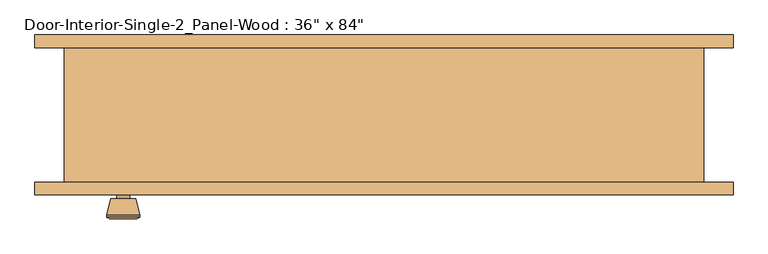
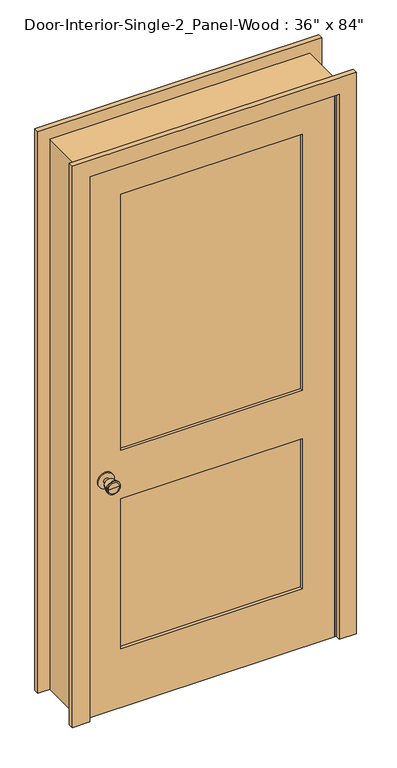
"""IFC4 building model written with IfcOpenShell, lengths in millimetres: door geometry."""

from ifc_helpers import new_model, si_unit, point, frame, frame_2d, origin, place, context, project, spatial, polyline, circle_curve, trimmed, segment, composite_curve, outline, extrude, faceted_brep, source, transform, mapped, element, save
from ifc_brep_helpers import plane_surface, cylinder_surface, revolved_surface, advanced_brep


def door_387d6dd4(model_context):
    return source(origin(), model_context, "Body", "SolidModel", [
        advanced_brep(
        [(-393.7, -57.5, 914.4), (-403.7, -57.5, 914.4), (-383.7, -57.5, 914.4), (-373.2241324, -8.5, 914.4), (-414.1758676, -8.5, 914.4), (-393.7, -8.5, 914.4), (-368.7, -10.3278681, 914.4), (-418.7, -10.3278681, 914.4), (-368.7, -13.7915463, 914.4), (-418.7, -13.7915463, 914.4), (-375.063764, -38.5, 914.4), (-412.336236, -38.5, 914.4), (-383.7, -38.5, 914.4), (-403.7, -38.5, 914.4)],
        [
            (0, 1),
            (1, 2, circle_curve(frame((-393.7, -57.5, 914.4), z_axis=(0.0, -1.0, 0.0), x_axis=(-1.0, 0.0, 0.0)), 10.0)),
            (2, 0),
            (2, 1, circle_curve(frame((-393.7, -57.5, 914.4), z_axis=(0.0, -1.0, 0.0), x_axis=(-1.0, 0.0, 0.0)), 10.0)),
            (3, 4, circle_curve(frame((-393.7, -8.5, 914.4), z_axis=(0.0, 1.0, 0.0), x_axis=(-1.0, 0.0, 0.0)), 20.4758676)),
            (4, 5),
            (5, 3),
            (4, 3, circle_curve(frame((-393.7, -8.5, 914.4), z_axis=(0.0, 1.0, 0.0), x_axis=(-1.0, 0.0, 0.0)), 20.4758676)),
            (6, 7, circle_curve(frame((-393.7, -10.3278681, 914.4), z_axis=(0.0, 1.0, 0.0), x_axis=(-1.0, 0.0, 0.0)), 25.0)),
            (7, 4),
            (3, 6),
            (7, 6, circle_curve(frame((-393.7, -10.3278681, 914.4), z_axis=(0.0, 1.0, 0.0), x_axis=(-1.0, 0.0, 0.0)), 25.0)),
            (8, 9, circle_curve(frame((-393.7, -13.7915463, 914.4), z_axis=(0.0, 1.0, 0.0), x_axis=(-1.0, 0.0, 0.0)), 25.0)),
            (9, 7),
            (6, 8),
            (9, 8, circle_curve(frame((-393.7, -13.7915463, 914.4), z_axis=(0.0, 1.0, 0.0), x_axis=(-1.0, 0.0, 0.0)), 25.0)),
            (10, 11, circle_curve(frame((-393.7, -38.5, 914.4), z_axis=(0.0, 1.0, 0.0), x_axis=(-1.0, 0.0, 0.0)), 18.636236)),
            (11, 9),
            (8, 10),
            (11, 10, circle_curve(frame((-393.7, -38.5, 914.4), z_axis=(0.0, 1.0, 0.0), x_axis=(-1.0, 0.0, 0.0)), 18.636236)),
            (12, 13, circle_curve(frame((-393.7, -38.5, 914.4), z_axis=(0.0, 1.0, 0.0), x_axis=(-1.0, 0.0, 0.0)), 10.0)),
            (13, 11),
            (10, 12),
            (13, 12, circle_curve(frame((-393.7, -38.5, 914.4), z_axis=(0.0, 1.0, 0.0), x_axis=(-1.0, 0.0, 0.0)), 10.0)),
            (1, 13),
            (12, 2),
        ],
        [
            plane_surface(frame((-393.7, -57.5, 914.4), z_axis=(0.0, -1.0, 0.0), x_axis=(-1.0, 0.0, 0.0))),
            plane_surface(frame((-393.7, -8.5, 914.4), z_axis=(0.0, 1.0, 0.0), x_axis=(-1.0, 0.0, 0.0))),
            revolved_surface(polyline([(-414.1758676, -8.5, 914.4), (-418.7, -10.3278681, 914.4)]), (-393.7, -57.5, 914.4), (0.0, -1.0, 0.0)),
            cylinder_surface(frame((-393.7, -57.5, 914.4), z_axis=(0.0, -1.0, 0.0), x_axis=(-1.0, 0.0, 0.0)), 25.0),
            revolved_surface(polyline([(-418.7, -13.7915463, 914.4), (-412.336236, -38.5, 914.4)]), (-393.7, -57.5, 914.4), (0.0, -1.0, 0.0)),
            plane_surface(frame((-393.7, -38.5, 914.4), z_axis=(0.0, -1.0, 0.0), x_axis=(-1.0, 0.0, 0.0))),
            cylinder_surface(frame((-393.7, -57.5, 914.4), z_axis=(0.0, -1.0, 0.0), x_axis=(-1.0, 0.0, 0.0)), 10.0),
        ],
        [
            (0, [[1, 2, 3]]),
            (0, [[-3, 4, -1]]),
            (1, [[5, 6, 7]]),
            (1, [[8, -7, -6]]),
            (2, [[9, 10, -5, 11]]),
            (2, [[12, -11, -8, -10]]),
            (3, [[13, 14, -9, 15]]),
            (3, [[16, -15, -12, -14]]),
            (4, [[17, 18, -13, 19]]),
            (4, [[20, -19, -16, -18]]),
            (5, [[21, 22, -17, 23]]),
            (5, [[24, -23, -20, -22]]),
            (6, [[-2, 25, -21, 26]]),
            (6, [[-4, -26, -24, -25]]),
        ],
    ),
        extrude(outline(composite_curve([segment(trimmed(circle_curve(frame_2d((914.4, -393.7)), 30.0), [point((914.4, -423.7))], [point((914.4, -363.7))], False, "CARTESIAN"), True, "CONTINUOUS"), segment(trimmed(circle_curve(frame_2d((914.4, -393.7)), 30.0), [point((914.4, -363.7))], [point((914.4, -423.7))], False, "CARTESIAN"), True, "CONTINUOUS")], self_intersect=False)), frame((0.0, -63.5, 0.0), z_axis=(0.0, 1.0, 0.0), x_axis=(0.0, 0.0, 1.0)), (0.0, 0.0, 1.0), 6.0),
        advanced_brep(
        [(-393.7, -104.425, 914.4), (-383.7, -104.425, 914.4), (-403.7, -104.425, 914.4), (-373.2241324, -153.425, 914.4), (-393.7, -153.425, 914.4), (-414.1758676, -153.425, 914.4), (-368.7, -151.5971319, 914.4), (-418.7, -151.5971319, 914.4), (-368.7, -148.1334537, 914.4), (-418.7, -148.1334537, 914.4), (-375.063764, -123.425, 914.4), (-412.336236, -123.425, 914.4), (-383.7, -123.425, 914.4), (-403.7, -123.425, 914.4)],
        [
            (0, 1),
            (1, 2, circle_curve(frame((-393.7, -104.425, 914.4), z_axis=(0.0, 1.0, 0.0), x_axis=(-1.0, 0.0, 0.0)), 10.0)),
            (2, 0),
            (2, 1, circle_curve(frame((-393.7, -104.425, 914.4), z_axis=(0.0, 1.0, 0.0), x_axis=(-1.0, 0.0, 0.0)), 10.0)),
            (3, 4),
            (4, 5),
            (5, 3, circle_curve(frame((-393.7, -153.425, 914.4), z_axis=(0.0, -1.0, 0.0), x_axis=(-1.0, 0.0, 0.0)), 20.4758676)),
            (3, 5, circle_curve(frame((-393.7, -153.425, 914.4), z_axis=(0.0, -1.0, 0.0), x_axis=(-1.0, 0.0, 0.0)), 20.4758676)),
            (6, 3),
            (5, 7),
            (7, 6, circle_curve(frame((-393.7, -151.5971319, 914.4), z_axis=(0.0, -1.0, 0.0), x_axis=(-1.0, 0.0, 0.0)), 25.0)),
            (6, 7, circle_curve(frame((-393.7, -151.5971319, 914.4), z_axis=(0.0, -1.0, 0.0), x_axis=(-1.0, 0.0, 0.0)), 25.0)),
            (8, 6),
            (7, 9),
            (9, 8, circle_curve(frame((-393.7, -148.1334537, 914.4), z_axis=(0.0, -1.0, 0.0), x_axis=(-1.0, 0.0, 0.0)), 25.0)),
            (8, 9, circle_curve(frame((-393.7, -148.1334537, 914.4), z_axis=(0.0, -1.0, 0.0), x_axis=(-1.0, 0.0, 0.0)), 25.0)),
            (10, 8),
            (9, 11),
            (11, 10, circle_curve(frame((-393.7, -123.425, 914.4), z_axis=(0.0, -1.0, 0.0), x_axis=(-1.0, 0.0, 0.0)), 18.636236)),
            (10, 11, circle_curve(frame((-393.7, -123.425, 914.4), z_axis=(0.0, -1.0, 0.0), x_axis=(-1.0, 0.0, 0.0)), 18.636236)),
            (12, 10),
            (11, 13),
            (13, 12, circle_curve(frame((-393.7, -123.425, 914.4), z_axis=(0.0, -1.0, 0.0), x_axis=(-1.0, 0.0, 0.0)), 10.0)),
            (12, 13, circle_curve(frame((-393.7, -123.425, 914.4), z_axis=(0.0, -1.0, 0.0), x_axis=(-1.0, 0.0, 0.0)), 10.0)),
            (1, 12),
            (13, 2),
        ],
        [
            plane_surface(frame((-393.7, -104.425, 914.4), z_axis=(0.0, 1.0, 0.0), x_axis=(-1.0, 0.0, 0.0))),
            plane_surface(frame((-393.7, -153.425, 914.4), z_axis=(0.0, -1.0, 0.0), x_axis=(-1.0, 0.0, 0.0))),
            revolved_surface(polyline([(-414.1758676, -153.425, 914.4), (-418.7, -151.5971319, 914.4)]), (-393.7, -104.425, 914.4), (0.0, 1.0, 0.0)),
            cylinder_surface(frame((-393.7, -104.425, 914.4), z_axis=(0.0, 1.0, 0.0), x_axis=(-1.0, 0.0, 0.0)), 25.0),
            revolved_surface(polyline([(-418.7, -148.1334537, 914.4), (-412.336236, -123.425, 914.4)]), (-393.7, -104.425, 914.4), (0.0, 1.0, 0.0)),
            plane_surface(frame((-393.7, -123.425, 914.4), z_axis=(0.0, 1.0, 0.0), x_axis=(-1.0, 0.0, 0.0))),
            cylinder_surface(frame((-393.7, -104.425, 914.4), z_axis=(0.0, 1.0, 0.0), x_axis=(-1.0, 0.0, 0.0)), 10.0),
        ],
        [
            (0, [[1, 2, 3]]),
            (0, [[-3, 4, -1]]),
            (1, [[5, 6, 7]]),
            (1, [[-6, -5, 8]]),
            (2, [[9, -7, 10, 11]]),
            (2, [[-10, -8, -9, 12]]),
            (3, [[13, -11, 14, 15]]),
            (3, [[-14, -12, -13, 16]]),
            (4, [[17, -15, 18, 19]]),
            (4, [[-18, -16, -17, 20]]),
            (5, [[21, -19, 22, 23]]),
            (5, [[-22, -20, -21, 24]]),
            (6, [[25, -23, 26, -2]]),
            (6, [[-26, -24, -25, -4]]),
        ],
    ),
        extrude(outline(composite_curve([segment(trimmed(circle_curve(frame_2d((914.4, -393.7)), 30.0), [point((914.4, -423.7))], [point((914.4, -363.7))], False, "CARTESIAN"), True, "CONTINUOUS"), segment(trimmed(circle_curve(frame_2d((914.4, -393.7)), 30.0), [point((914.4, -363.7))], [point((914.4, -423.7))], False, "CARTESIAN"), True, "CONTINUOUS")], self_intersect=False)), frame((0.0, -104.425, 0.0), z_axis=(0.0, 1.0, 0.0), x_axis=(0.0, 0.0, 1.0)), (0.0, 0.0, 1.0), 6.0),
        extrude(outline(polyline([(336.55, -75.1416667), (336.55, -86.7833333), (-336.55, -86.7833333), (-336.55, -75.1416667), (336.55, -75.1416667)])), frame((0.0, 0.0, 1009.65), z_axis=(0.0, 0.0, 1.0), x_axis=(1.0, 0.0, 0.0)), (0.0, 0.0, 1.0), 1004.8875),
        extrude(outline(polyline([(336.55, -75.1416667), (336.55, -86.7833333), (-336.55, -86.7833333), (-336.55, -75.1416667), (336.55, -75.1416667)])), frame((0.0, 0.0, 231.775), z_axis=(0.0, 0.0, 1.0), x_axis=(1.0, 0.0, 0.0)), (0.0, 0.0, 1.0), 587.375),
        extrude(outline(polyline([(2133.6, -457.2), (0.0, -457.2), (0.0, 457.2), (2133.6, 457.2), (2133.6, -457.2)]), holes=[polyline([(2014.5375, -336.55), (2014.5375, 336.55), (1009.65, 336.55), (1009.65, -336.55), (2014.5375, -336.55)]), polyline([(819.15, -336.55), (819.15, 336.55), (231.775, 336.55), (231.775, -336.55), (819.15, -336.55)])]), frame((0.0, -98.425, 0.0), z_axis=(0.0, 1.0, 0.0), x_axis=(0.0, 0.0, 1.0)), (0.0, 0.0, 1.0), 34.925),
        faceted_brep([(482.6, -98.425, 0.0), (457.2, -98.425, 0.0), (457.2, -63.5, 0.0), (444.5, -63.5, 0.0), (444.5, -28.575, 0.0), (457.2, -28.575, 0.0), (457.2, 104.775, 0.0), (482.6, 104.775, 0.0), (482.6, 104.775, 2159.0), (482.6, -98.425, 2159.0), (457.2, 104.775, 2133.6), (-457.2, 104.775, 2133.6), (-457.2, 104.775, 0.0), (-482.6, 104.775, 0.0), (-482.6, 104.775, 2159.0), (457.2, -28.575, 2133.6), (444.5, -28.575, 2120.9), (-444.5, -28.575, 2120.9), (-444.5, -28.575, 0.0), (-457.2, -28.575, 0.0), (-457.2, -28.575, 2133.6), (444.5, -63.5, 2120.9), (457.2, -63.5, 2133.6), (-457.2, -63.5, 2133.6), (-457.2, -63.5, 0.0), (-444.5, -63.5, 0.0), (-444.5, -63.5, 2120.9), (457.2, -98.425, 2133.6), (-482.6, -98.425, 2159.0), (-482.6, -98.425, 0.0), (-457.2, -98.425, 0.0), (-457.2, -98.425, 2133.6)], [[[0, 1, 2, 3, 4, 5, 6, 7]], [[7, 8, 9, 0]], [[6, 10, 11, 12, 13, 14, 8, 7]], [[5, 15, 10, 6]], [[4, 16, 17, 18, 19, 20, 15, 5]], [[3, 21, 16, 4]], [[2, 22, 23, 24, 25, 26, 21, 3]], [[1, 27, 22, 2]], [[0, 9, 28, 29, 30, 31, 27, 1]], [[8, 14, 28, 9]], [[15, 20, 11, 10]], [[21, 26, 17, 16]], [[27, 31, 23, 22]], [[29, 13, 12, 19, 18, 25, 24, 30]], [[14, 13, 29, 28]], [[20, 19, 12, 11]], [[26, 25, 18, 17]], [[31, 30, 24, 23]]]),
        extrude(outline(polyline([(0.0, 527.05), (2203.45, 527.05), (2203.45, -527.05), (0.0, -527.05), (0.0, -463.55), (2139.95, -463.55), (2139.95, 463.55), (0.0, 463.55), (0.0, 527.05)])), frame((0.0, 104.775, 0.0), z_axis=(0.0, 1.0, 0.0), x_axis=(0.0, 0.0, 1.0)), (0.0, 0.0, 1.0), 19.05),
        extrude(outline(polyline([(0.0, 527.05), (2203.45, 527.05), (2203.45, -527.05), (0.0, -527.05), (0.0, -463.55), (2139.95, -463.55), (2139.95, 463.55), (0.0, 463.55), (0.0, 527.05)])), frame((0.0, -117.475, 0.0), z_axis=(0.0, 1.0, 0.0), x_axis=(0.0, 0.0, 1.0)), (0.0, 0.0, 1.0), 19.05),
    ])


if __name__ == "__main__":
    model = new_model("IFC4")
    model_context = context("Model", 3, world=origin())
    ifc_project = project(units=[si_unit("LENGTHUNIT", "METRE", prefix="MILLI")], contexts=[model_context])
    site = spatial("IfcSite", under=ifc_project)
    building = spatial("IfcBuilding", under=site)
    placement = place(None, origin())
    door_shape = door_387d6dd4(model_context)
    element("IfcDoor", 1, ObjectType="Door-Interior-Single-2_Panel-Wood : 36\" x 84\"", at=placement, inside=building, context=model_context, shape_type="MappedRepresentation", body=[
        mapped(door_shape, transform((0.0, 0.0, 0.0), x_axis=(1.0, 0.0, 0.0), y_axis=(0.0, 1.0, 0.0), z_axis=(0.0, 0.0, 1.0))),
    ])
    save(model, "model.ifc")

# Revit data of these elements
# Type "Door-Interior-Single-2_Panel-Wood : 36\" x 84\""
#   Type Mark = "11"
#   Assembly Code = "C1020300"
#   Analytic Construction = "Wooden"
#   Top Rail = 0' - 4 11/16"
#   Thickness = 0' - 1 3/8"
#   Thermal Resistance (R) = 2.5876 (h·ft²·°F)/BTU
#   Swing Angle [instance default] = 90.00°
#   Stiles = 0' - 4 3/4"
#   Rough Width = 3' - 2"
#   Rough Height = 7' - 1"
#   Lock Rail = 0' - 7 1/2"
#   Height = 7' - 0"
#   Width = 3' - 0"
#   Heat Transfer Coefficient (U) = 0.3865 BTU/(h·ft²·°F)
#   Bottom Rail = 0' - 9 1/8"
#   Trim Material = Cherry
#   Panel Material = Cherry
#   Frame Material = Cherry
#   Door Handle Material = Aluminum
#   Visual Light Transmittance = 0
#   Solar Heat Gain Coefficient = 0
#   Wall Closure = (empty or 0)
#   Function = (empty or 0)
# Element 1 (IfcDoor, "Door-Interior-Single-2_Panel-Wood : 36\" x 84\"")
#   Materials on its faces: "Cherry", "Aluminum"
# Materials
#   "Cherry": class "Wood", colour RGB 226 177 128, transparency 0, Description = "Prunus Serotina", Cost = 0
#   "Aluminum": class "Metal", colour RGB 247 247 247, transparency 0, Description = "Aluminum 6061", Cost = 0
